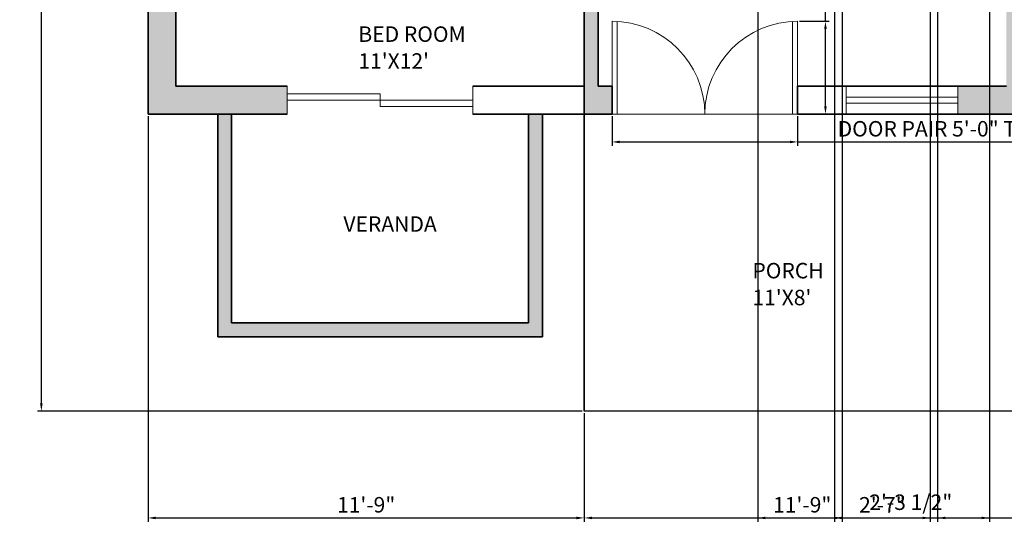
# Model space of a CAD drawing. Units: inches. Extents: x 2923 to 3500, y 1684 to 2381.
# Tile 1 of 12: x 2928 to 3246, y 1684 to 1848. Entities that reach past the tile are written whole.
import ezdxf

# ---------------------------------------------------------------- set-up
doc = ezdxf.new("R2010")
doc.units = ezdxf.units.IN
for name, color, linetype, lineweight in [('A-ANNO-DIMS', 2, 'Continuous', 18), ('A-AREA-IDEN', 7, 'Continuous', 18), ('A-DOOR', 3, 'Continuous', 18), ('A-FLOR-OTLN', 7, 'Continuous', 25), ('A-GLAZ', 4, 'Continuous', 18), ('A-WALL', 7, 'Continuous', 35), ('A-WALL-PATT', 9, 'Continuous', 13)]:
    doc.layers.add(name, color=color, linetype=linetype, lineweight=lineweight)
doc.styles.get("Standard").update_dxf_attribs({"font": 'txt', "height": 5})
doc.dimstyles.new('ISO-25', dxfattribs={"dimtxt": 5, "dimasz": 2.5, "dimexe": 1.25, "dimexo": 0.625, "dimtad": 1, "dimlunit": 3, "dimtxsty": 'Standard', "dimcen": 2.5, "dimadec": 0, "dimazin": 0, "dimtfac": 1, "dimtmove": 0, "dimatfit": 3, "dimfxl": 1, "dimarcsym": 0})

# ---------------------------------------------------------------- blocks, each defined once
blk = doc.blocks.new('DOOR-PAIR-60IN')
for p, q in [((0, 30), (0, 0)), ((1.67, 29.95), (1.67, 0)), ((58.33, 29.95), (58.33, 0)), ((60, 30), (60, 0)), ((0, 0), (30, 0)), ((60, 0), (30, 0))]:
    blk.add_line(p, q)
for centre, start, end in [((0, 0), 0, 90), ((60, 0), 90, 180)]:
    blk.add_arc(centre, 30, start, end)
blk = doc.blocks.new('WINDOW-36IN')
for p, q in [((36, 9), (0, 9)), ((0, 9), (0, 0)), ((36, 0), (36, 9)), ((36, 5.5), (0, 5.5)), ((36, 3.5), (0, 3.5)), ((0, 0), (36, 0))]:
    blk.add_line(p, q)
blk = doc.blocks.new('WINDOW-SLIDING-60IN')
for p, q in [((0, 0), (0, 9)), ((30, 4.5), (30, 6.5)), ((30, 6.5), (60, 6.5)), ((60, 0), (60, 9)), ((60, 4.5), (0, 4.5)), ((30, 4.5), (30, 2.5)), ((30, 2.5), (0, 2.5))]:
    blk.add_line(p, q)
blk = doc.blocks.new('VERANDA-PARAPET')
for p, q in [((0, 72), (0, 0)), ((4.5, 72), (4.5, 4.5)), ((100.5, 72), (100.5, 4.5)), ((105, 72), (105, 0)), ((100.5, 4.5), (4.5, 4.5)), ((105, 0), (0, 0))]:
    blk.add_line(p, q)
blk = doc.blocks.new('*D29')
at = {"layer": 'A-ANNO-DIMS', "color": 0, "lineweight": -2, "transparency": 16777216}
for p, q in [((3119.23, 1816.78), (3119.23, 1807.16)), ((3179.23, 1816.78), (3179.23, 1807.16)), ((3121.73, 1808.41), (3176.73, 1808.41)), ((3179.23, 1808.41), (3270.12, 1808.41))]:
    blk.add_line(p, q, dxfattribs=at)
at = {"layer": 'A-ANNO-DIMS', "color": 0, "transparency": 16777216}
for points in [[(3121.73, 1808.82), (3121.73, 1807.99), (3119.23, 1808.41)], [(3176.73, 1808.82), (3176.73, 1807.99), (3179.23, 1808.41)]]:
    blk.add_solid(points, dxfattribs=at)
at = {"layer": 'Defpoints', "color": 0, "transparency": 16777216}
for p in [(3119.23, 1817.41), (3179.23, 1817.41), (3179.23, 1808.41)]:
    blk.add_point(p, dxfattribs=at)
at = {"layer": 'A-ANNO-DIMS', "color": 0, "transparency": 16777216, "insert": (3225.93, 1812.01), "char_height": 5, "attachment_point": 5}
blk.add_mtext('DOOR PAIR 5\'-0" TYP.', dxfattribs=at)
blk = doc.blocks.new('*D30')
at = {"layer": 'A-ANNO-DIMS', "color": 0, "lineweight": -2, "transparency": 16777216}
for p, q in [((3188.23, 1847.41), (3188.23, 1891.63)), ((3179.85, 1847.41), (3189.48, 1847.41)), ((3188.23, 1819.91), (3188.23, 1844.91)), ((3179.85, 1817.41), (3189.48, 1817.41))]:
    blk.add_line(p, q, dxfattribs=at)
at = {"layer": 'A-ANNO-DIMS', "color": 0, "transparency": 16777216}
for points in [[(3187.81, 1844.91), (3188.65, 1844.91), (3188.23, 1847.41)], [(3187.81, 1819.91), (3188.65, 1819.91), (3188.23, 1817.41)]]:
    blk.add_solid(points, dxfattribs=at)
at = {"layer": 'Defpoints', "color": 0, "transparency": 16777216}
for p in [(3179.23, 1847.41), (3188.23, 1847.41), (3179.23, 1817.41)]:
    blk.add_point(p, dxfattribs=at)
at = {"layer": 'A-ANNO-DIMS', "color": 0, "transparency": 16777216, "insert": (3184.63, 1870.77), "char_height": 5, "attachment_point": 5, "rotation": 90}
blk.add_mtext('2\'-6" TYP.', dxfattribs=at)
blk = doc.blocks.new('*D50')
at = {"layer": 'A-ANNO-DIMS', "color": 0, "lineweight": -2, "transparency": 16777216}
for p, q in [((2991.1, 2334.41), (2933.48, 2334.41)), ((2934.73, 1723.91), (2934.73, 2331.91)), ((3109.6, 1721.41), (2933.48, 1721.41))]:
    blk.add_line(p, q, dxfattribs=at)
at = {"layer": 'A-ANNO-DIMS', "color": 0, "transparency": 16777216}
for points in [[(2934.31, 2331.91), (2935.15, 2331.91), (2934.73, 2334.41)], [(2934.31, 1723.91), (2935.15, 1723.91), (2934.73, 1721.41)]]:
    blk.add_solid(points, dxfattribs=at)
at = {"layer": 'Defpoints', "color": 0, "transparency": 16777216}
for p in [(2934.73, 2334.41), (2991.73, 2334.41), (3110.23, 1721.41)]:
    blk.add_point(p, dxfattribs=at)
at = {"layer": 'A-ANNO-DIMS', "color": 0, "transparency": 16777216, "insert": (2931.13, 2027.91), "char_height": 5, "attachment_point": 5, "rotation": 90}
blk.add_mtext('51\'-1"', dxfattribs=at)
blk = doc.blocks.new('*D54')
at = {"layer": 'A-ANNO-DIMS', "color": 0, "lineweight": -2, "transparency": 16777216}
for p, q in [((3166.32, 2236.75), (3166.32, 1685.66)), ((3193.64, 2236.75), (3193.64, 1685.66)), ((3168.82, 1686.91), (3191.14, 1686.91)), ((3193.64, 1686.91), (3235.49, 1686.91))]:
    blk.add_line(p, q, dxfattribs=at)
at = {"layer": 'A-ANNO-DIMS', "color": 0, "transparency": 16777216}
for points in [[(3168.82, 1687.32), (3168.82, 1686.49), (3166.32, 1686.91)], [(3191.14, 1687.32), (3191.14, 1686.49), (3193.64, 1686.91)]]:
    blk.add_solid(points, dxfattribs=at)
at = {"layer": 'Defpoints', "color": 0, "transparency": 16777216}
for p in [(3166.32, 2237.38), (3193.64, 2237.38), (3193.64, 1686.91)]:
    blk.add_point(p, dxfattribs=at)
at = {"layer": 'A-ANNO-DIMS', "color": 0, "transparency": 16777216, "insert": (3215.82, 1691.34), "char_height": 5, "attachment_point": 5}
blk.add_mtext('2\'-3 1/2"', dxfattribs=at)
blk = doc.blocks.new('*D61')
at = {"layer": 'A-ANNO-DIMS', "color": 0, "lineweight": -2, "transparency": 16777216}
for p, q in [((3224.5, 1890.49), (3224.5, 1685.66)), ((3241.23, 1890.49), (3241.23, 1685.66)), ((3227, 1686.91), (3238.73, 1686.91)), ((3241.23, 1686.91), (3282.12, 1686.91))]:
    blk.add_line(p, q, dxfattribs=at)
at = {"layer": 'A-ANNO-DIMS', "color": 0, "transparency": 16777216}
for points in [[(3227, 1687.32), (3227, 1686.49), (3224.5, 1686.91)], [(3238.73, 1687.32), (3238.73, 1686.49), (3241.23, 1686.91)]]:
    blk.add_solid(points, dxfattribs=at)
at = {"layer": 'Defpoints', "color": 0, "transparency": 16777216}
for p in [(3224.5, 1891.12), (3241.23, 1891.12), (3241.23, 1686.91)]:
    blk.add_point(p, dxfattribs=at)
at = {"layer": 'A-ANNO-DIMS', "color": 0, "transparency": 16777216, "insert": (3262.92, 1691.34), "char_height": 5, "attachment_point": 5}
blk.add_mtext('1\'-4 1/2"', dxfattribs=at)
blk = doc.blocks.new('*D64')
at = {"layer": 'A-ANNO-DIMS', "color": 0, "lineweight": -2, "transparency": 16777216}
for p, q in [((3191.11, 1865.68), (3191.11, 1685.66)), ((3222.14, 1865.68), (3222.14, 1685.66)), ((3193.61, 1686.91), (3219.64, 1686.91))]:
    blk.add_line(p, q, dxfattribs=at)
at = {"layer": 'A-ANNO-DIMS', "color": 0, "transparency": 16777216}
for points in [[(3193.61, 1687.32), (3193.61, 1686.49), (3191.11, 1686.91)], [(3219.64, 1687.32), (3219.64, 1686.49), (3222.14, 1686.91)]]:
    blk.add_solid(points, dxfattribs=at)
at = {"layer": 'Defpoints', "color": 0, "transparency": 16777216}
for p in [(3191.11, 1866.31), (3222.14, 1866.31), (3222.14, 1686.91)]:
    blk.add_point(p, dxfattribs=at)
at = {"layer": 'A-ANNO-DIMS', "color": 0, "transparency": 16777216, "insert": (3206.63, 1690.51), "char_height": 5, "attachment_point": 5}
blk.add_mtext('2\'-7"', dxfattribs=at)
blk = doc.blocks.new('*D68')
at = {"layer": 'A-ANNO-DIMS', "color": 0, "lineweight": -2, "transparency": 16777216}
for p, q in [((2969.23, 1816.78), (2969.23, 1685.66)), ((3110.23, 1720.78), (3110.23, 1685.66)), ((2971.73, 1686.91), (3107.73, 1686.91))]:
    blk.add_line(p, q, dxfattribs=at)
at = {"layer": 'A-ANNO-DIMS', "color": 0, "transparency": 16777216}
for points in [[(2971.73, 1687.32), (2971.73, 1686.49), (2969.23, 1686.91)], [(3107.73, 1687.32), (3107.73, 1686.49), (3110.23, 1686.91)]]:
    blk.add_solid(points, dxfattribs=at)
at = {"layer": 'Defpoints', "color": 0, "transparency": 16777216}
for p in [(2969.23, 1817.41), (3110.23, 1721.41), (3110.23, 1686.91)]:
    blk.add_point(p, dxfattribs=at)
at = {"layer": 'A-ANNO-DIMS', "color": 0, "transparency": 16777216, "insert": (3039.73, 1690.51), "char_height": 5, "attachment_point": 5}
blk.add_mtext('11\'-9"', dxfattribs=at)
blk = doc.blocks.new('*D69')
at = {"layer": 'A-ANNO-DIMS', "color": 0, "lineweight": -2, "transparency": 16777216}
for p, q in [((3110.23, 1720.78), (3110.23, 1685.66)), ((3251.23, 1720.78), (3251.23, 1685.66)), ((3112.73, 1686.91), (3248.73, 1686.91))]:
    blk.add_line(p, q, dxfattribs=at)
at = {"layer": 'A-ANNO-DIMS', "color": 0, "transparency": 16777216}
for points in [[(3112.73, 1687.32), (3112.73, 1686.49), (3110.23, 1686.91)], [(3248.73, 1687.32), (3248.73, 1686.49), (3251.23, 1686.91)]]:
    blk.add_solid(points, dxfattribs=at)
at = {"layer": 'Defpoints', "color": 0, "transparency": 16777216}
for p in [(3110.23, 1721.41), (3251.23, 1721.41), (3251.23, 1686.91)]:
    blk.add_point(p, dxfattribs=at)
at = {"layer": 'A-ANNO-DIMS', "color": 0, "transparency": 16777216, "insert": (3180.73, 1690.51), "char_height": 5, "attachment_point": 5}
blk.add_mtext('11\'-9"', dxfattribs=at)

msp = doc.modelspace()

# ---------------------------------------------------------------- hatches: boundary and pattern name
at = {"layer": 'A-WALL-PATT'}
h = msp.add_hatch(color=256, dxfattribs=at)
h.dxf.hatch_style = 1
h.paths.add_polyline_path([(3014.23, 2262.406), (2969.23, 2262.406), (2969.23, 2201.5), (2978.23, 2201.5), (2978.23, 2213.699), (2978.23, 2253.406), (3014.23, 2253.406)])
h.paths.add_polyline_path([(3119.23, 2262.406), (3074.23, 2262.406), (3074.23, 2253.406), (3110.23, 2253.406), (3110.23, 2109.406), (3105.73, 2109.406), (3105.73, 2104.906), (3114.73, 2104.906), (3114.73, 2152.906), (3119.23, 2152.906), (3119.23, 2157.406), (3114.73, 2157.406), (3114.73, 2253.406), (3119.23, 2253.406)])
h.paths.add_polyline_path([(3179.98, 2262.406), (3149.23, 2262.406), (3149.23, 2253.406), (3179.98, 2253.406)], flags=0)
h.paths.add_polyline_path([(3295.73, 2262.406), (3215.98, 2262.406), (3215.98, 2253.406), (3246.73, 2253.406), (3246.73, 2157.406), (3149.23, 2157.406), (3149.23, 2152.906), (3246.73, 2152.906), (3246.73, 2149.906), (3251.23, 2149.906), (3251.23, 2253.406), (3295.73, 2253.406)])
h.paths.add_polyline_path([(3397.23, 2262.406), (3343.73, 2262.406), (3343.73, 2253.406), (3349.929, 2253.406), (3388.23, 2253.406), (3388.23, 2199.406), (3397.23, 2199.406)])
h.paths.add_polyline_path([(3369.935, 2334.406), (3264.935, 2334.406), (3264.935, 2262.406), (3269.435, 2262.406), (3269.435, 2329.906), (3365.435, 2329.906), (3365.435, 2262.406), (3369.935, 2262.406)])
h.paths.add_polyline_path([(3096.73, 2334.406), (2991.73, 2334.406), (2991.73, 2262.406), (2996.23, 2262.406), (2996.23, 2329.906), (3092.23, 2329.906), (3092.23, 2262.406), (3096.73, 2262.406)])
h.paths.add_polyline_path([(3397.23, 2163.406), (3388.23, 2163.406), (3388.23, 2109.406), (3251.23, 2109.406), (3251.23, 2113.906), (3246.73, 2113.906), (3246.73, 2092.906), (3251.23, 2092.906), (3251.23, 2104.906), (3435.23, 2104.906), (3435.23, 2080.906), (3444.23, 2080.906), (3444.23, 2109.406), (3397.23, 2109.406)])
h.paths.add_polyline_path([(3444.23, 2044.906), (3435.23, 2044.906), (3435.23, 2020.906), (3251.23, 2020.906), (3251.23, 2032.906), (3246.73, 2032.906), (3246.73, 2016.406), (3251.23, 2016.406), (3287.73, 2016.406), (3287.73, 1968.406), (3287.23, 1968.406), (3287.23, 1963.906), (3296.73, 1963.906), (3296.73, 1968.406), (3292.23, 1968.406), (3292.23, 2016.406), (3388.23, 2016.406), (3388.23, 2004.398), (3397.23, 2004.398), (3397.23, 2016.406), (3444.23, 2016.406)])
h.paths.add_polyline_path([(3397.23, 1980.398), (3388.23, 1980.398), (3388.23, 1979.998), (3388.23, 1969.828), (3388.23, 1968.406), (3326.73, 1968.406), (3326.73, 1963.906), (3388.23, 1963.906), (3388.23, 1913.156), (3397.23, 1913.156)])
h.paths.add_polyline_path([(3251.23, 1968.406), (3150.73, 1968.406), (3150.73, 1963.906), (3246.73, 1963.906), (3246.73, 1826.406), (3230.98, 1826.406), (3230.98, 1817.406), (3251.23, 1817.406), (3251.23, 1963.906)])
h.paths.add_polyline_path([(3114.73, 1968.406), (3105.73, 1968.406), (3105.73, 1963.906), (3110.23, 1963.906), (3110.23, 1817.406), (3119.23, 1817.406), (3119.23, 1826.406), (3114.73, 1826.406)])
h.paths.add_polyline_path([(3069.73, 1968.406), (3066.73, 1968.406), (3066.73, 1972.906), (3062.23, 1972.906), (3062.23, 1968.406), (2978.23, 1968.406), (2978.23, 1989.406), (2969.23, 1989.406), (2969.23, 1912.505), (2978.23, 1912.505), (2978.23, 1925.355), (2978.23, 1963.906), (3069.73, 1963.906)])
h.paths.add_polyline_path([(3066.73, 2104.906), (3069.73, 2104.906), (3069.73, 2109.406), (3057.73, 2109.406), (3057.73, 2104.906), (3062.23, 2104.906), (3062.23, 2038.906), (2978.23, 2038.906), (2978.23, 2059.906), (2969.23, 2059.906), (2969.23, 2013.406), (2978.23, 2013.406), (2978.23, 2034.406), (3062.23, 2034.406), (3062.23, 2002.906), (3066.73, 2002.906)])
h.paths.add_polyline_path([(3027.73, 2109.406), (2978.23, 2109.406), (2978.23, 2165.5), (2969.23, 2165.5), (2969.23, 2083.906), (2978.23, 2083.906), (2978.23, 2104.906), (3027.73, 2104.906)])
h.paths.add_polyline_path([(2978.23, 1876.505), (2969.23, 1876.505), (2969.23, 1817.406), (3014.23, 1817.406), (3014.23, 1826.406), (2978.23, 1826.406)])
h.paths.add_polyline_path([(2996.23, 1817.406), (2991.73, 1817.406), (2991.73, 1745.406), (3096.73, 1745.406), (3096.73, 1817.406), (3092.23, 1817.406), (3092.23, 1749.906), (2996.23, 1749.906)])
h.paths.add_polyline_path([(3289.73, 1826.406), (3251.23, 1826.406), (3251.23, 1817.406), (3289.73, 1817.406)])
h.paths.add_polyline_path([(3397.23, 1877.156), (3388.23, 1877.156), (3388.23, 1864.957), (3388.23, 1826.406), (3349.73, 1826.406), (3349.73, 1817.406), (3397.23, 1817.406)])
h.paths.add_polyline_path([(3374.267, 1817.406), (3369.767, 1817.406), (3369.767, 1749.906), (3273.767, 1749.906), (3273.767, 1817.406), (3269.267, 1817.406), (3269.267, 1745.406), (3374.267, 1745.406)])

# ---------------------------------------------------------------- linework, layer by layer
at = {"layer": 'A-FLOR-OTLN'}
msp.add_line((3251.23, 1721.406), (3110.23, 1721.406), dxfattribs=at)
at = {"layer": 'A-GLAZ'}
msp.add_line((3044.23, 1823.906), (3044.23, 1819.906), dxfattribs=at)
at = {"layer": 'A-WALL'}
for p, q in [((2969.23, 1817.406), (2969.23, 2262.406)), ((3114.73, 1826.406), (3114.73, 1968.406)), ((2978.23, 1826.406), (2978.23, 1963.906)), ((3110.23, 1721.406), (3110.23, 1963.906)), ((3014.23, 1826.406), (2978.23, 1826.406)), ((3110.23, 1826.406), (3074.23, 1826.406)), ((3119.23, 1826.406), (3114.73, 1826.406)), ((3119.23, 1826.406), (3119.23, 1817.406)), ((3246.73, 1826.406), (3179.23, 1826.406)), ((3179.23, 1826.406), (3179.23, 1817.406)), ((3014.23, 1817.406), (2969.23, 1817.406)), ((3119.23, 1817.406), (3074.23, 1817.406)), ((3289.73, 1817.406), (3179.23, 1817.406))]:
    msp.add_line(p, q, dxfattribs=at)

# ---------------------------------------------------------------- block references
at = {"layer": 'A-DOOR'}
msp.add_blockref('DOOR-PAIR-60IN', (3119.23, 1817.406), dxfattribs=at)
at = {"layer": 'A-GLAZ', "extrusion": (0, 0, -1), "zscale": -1}
msp.add_blockref('WINDOW-SLIDING-60IN', (-3074.23, 1817.406), dxfattribs=at)
at = {"layer": 'A-GLAZ'}
msp.add_blockref('WINDOW-36IN', (3194.98, 1817.406), dxfattribs=at)
at = {"layer": 'A-WALL'}
msp.add_blockref('VERANDA-PARAPET', (2991.73, 1745.406), dxfattribs=at)

# ---------------------------------------------------------------- texts
at = {"layer": 'A-AREA-IDEN'}
for s, p in [('BED ROOM', (3037.211, 1840.745)), ("11'X12'", (3037.211, 1832.06)), ('VERANDA', (3032.377, 1779.375)), ('PORCH', (3164.621, 1764.311)), ("11'X8'", (3164.621, 1755.626))]:
    msp.add_text(s, height=5, dxfattribs=at).set_placement(p)

# ---------------------------------------------------------------- dimensions: what is measured, and where the dimension line sits
at = {"layer": 'A-ANNO-DIMS'}
dim = msp.add_linear_dim(base=(2934.73, 2334.406), p1=(3110.23, 1721.406), p2=(2991.73, 2334.406), angle=90, dimstyle='ISO-25', override={"dimdec": 1, "dimlfac": 1, "dimrnd": 0, "dimzin": 1, "dimdsep": 46, "dimlunit": 4, "dimfrac": 2}, dxfattribs=at)
dim.commit()
dim.dimension.update_dxf_attribs({"geometry": '*D50', "text_midpoint": (2931.129, 2027.906)})
for base, p1, p2, picture, middle in [((3193.644, 1686.906), (3166.316, 2237.38), (3193.644, 2237.38), '*D54', (3215.817, 1691.341)), ((3241.226, 1686.906), (3224.497, 1891.115), (3241.226, 1891.115), '*D61', (3262.923, 1691.341)), ((3222.138, 1686.906), (3191.114, 1866.305), (3222.138, 1866.305), '*D64', (3206.626, 1690.507)), ((3110.23, 1686.906), (2969.23, 1817.406), (3110.23, 1721.406), '*D68', (3039.73, 1690.507)), ((3251.23, 1686.906), (3110.23, 1721.406), (3251.23, 1721.406), '*D69', (3180.73, 1690.507))]:
    dim = msp.add_linear_dim(base=base, p1=p1, p2=p2, dimstyle='ISO-25', override={"dimdec": 1, "dimlfac": 1, "dimrnd": 0, "dimzin": 1, "dimdsep": 46, "dimlunit": 4, "dimfrac": 2}, dxfattribs=at)
    dim.commit()
    dim.dimension.update_dxf_attribs({"geometry": picture, "text_midpoint": middle})
dim = msp.add_linear_dim(base=(3188.23, 1847.406), p1=(3179.23, 1817.406), p2=(3179.23, 1847.406), angle=90, text='<> TYP.', dimstyle='ISO-25', override={"dimdec": 1, "dimlfac": 1, "dimrnd": 0, "dimzin": 1, "dimdsep": 46, "dimlunit": 4, "dimfrac": 2}, dxfattribs=at)
dim.commit()
dim.dimension.update_dxf_attribs({"geometry": '*D30', "text_midpoint": (3184.629, 1870.769)})
dim = msp.add_linear_dim(base=(3179.23, 1808.406), p1=(3119.23, 1817.406), p2=(3179.23, 1817.406), text='DOOR PAIR <> TYP.', dimstyle='ISO-25', override={"dimdec": 1, "dimlfac": 1, "dimrnd": 0, "dimzin": 1, "dimdsep": 46, "dimlunit": 4, "dimfrac": 2}, dxfattribs=at)
dim.commit()
dim.dimension.update_dxf_attribs({"geometry": '*D29', "text_midpoint": (3225.926, 1812.007)})

doc.saveas('drawing.dxf')
